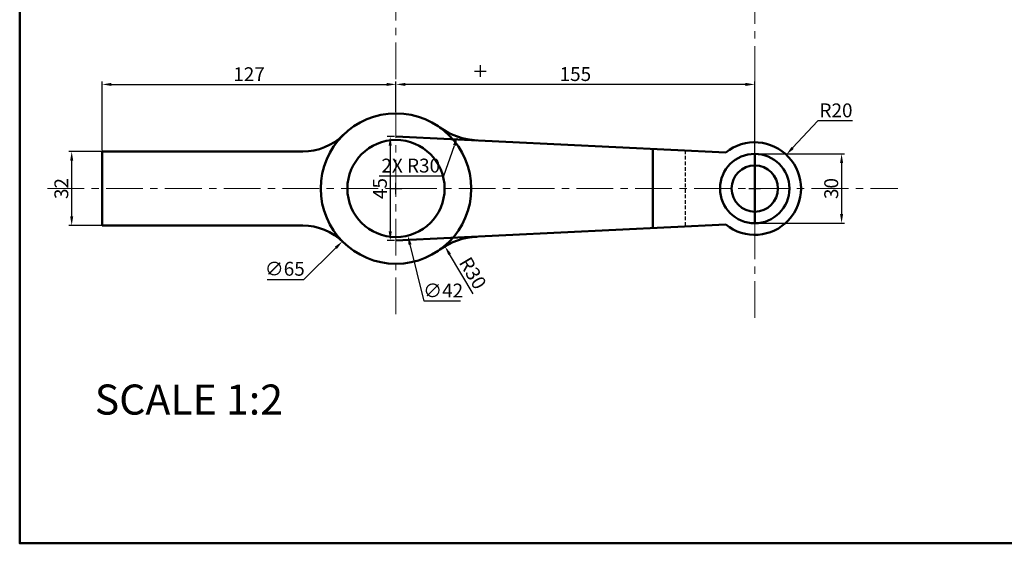
# Model space of a CAD drawing. Units: millimetres. Extents: x -1099 to -222, y 37 to 495.
# Tile 1 of 3: x -1099 to -674, y 37 to 263. Entities that reach past the tile are written whole.
import ezdxf

# ---------------------------------------------------------------- set-up
doc = ezdxf.new("R2010")
doc.units = ezdxf.units.MM
doc.header["$LTSCALE"] = 0.5
doc.linetypes.add('CENTER', pattern=[50.8, 31.75, -6.35, 6.35, -6.35])
doc.linetypes.add('HIDDEN', pattern=[9.525, 6.35, -3.175])
for name, color, linetype, lineweight in [('M-CNTR', 1, 'CENTER', 18), ('M-DIMS', 2, 'Continuous', 25), ('M-HIDN', 4, 'HIDDEN', 25), ('M-OUTL', 7, 'Continuous', 50), ('M-TEXT', 7, 'Continuous', 25), ('M-TTLB', 7, 'Continuous', 50)]:
    doc.layers.add(name, color=color, linetype=linetype, lineweight=lineweight)
doc.styles.get("Standard").update_dxf_attribs({"font": 'arial.ttf'})
doc.dimstyles.new('ISO-25', dxfattribs={"dimtxt": 6, "dimasz": 4, "dimexe": 1.25, "dimexo": 0.625, "dimtad": 1, "dimtoh": 1, "dimtxsty": 'Standard', "dimcen": 2.5, "dimadec": 0, "dimazin": 0, "dimtfac": 1, "dimtofl": 0, "dimtmove": 0, "dimatfit": 3, "dimfxl": 1, "dimarcsym": 0})

# ---------------------------------------------------------------- blocks, each defined once
blk = doc.blocks.new('*D1')
at = {"layer": 'Defpoints', "color": 0, "transparency": 16777216}
for p in [(-936.42, 234.94), (-936.42, 222.43), (-1063.42, 205.93)]:
    blk.add_point(p, dxfattribs=at)
at = {"layer": 'M-DIMS', "color": 0, "lineweight": -2, "transparency": 16777216}
for p, q in [((-1063.42, 206.56), (-1063.42, 236.19)), ((-1059.42, 234.94), (-940.42, 234.94)), ((-936.42, 223.06), (-936.42, 236.19))]:
    blk.add_line(p, q, dxfattribs=at)
at = {"layer": 'M-DIMS', "color": 0, "transparency": 16777216}
for points in [[(-1059.42, 235.6), (-1059.42, 234.27), (-1063.42, 234.94)], [(-940.42, 235.6), (-940.42, 234.27), (-936.42, 234.94)]]:
    blk.add_solid(points, dxfattribs=at)
at = {"layer": 'M-DIMS', "color": 0, "transparency": 16777216, "insert": (-999.92, 238.57), "char_height": 6, "attachment_point": 5}
blk.add_mtext('127', dxfattribs=at)
blk = doc.blocks.new('*D2')
at = {"layer": 'Defpoints', "color": 0, "transparency": 16777216}
for p in [(-936.42, 234.94), (-936.42, 222.43), (-781.42, 189.93)]:
    blk.add_point(p, dxfattribs=at)
at = {"layer": 'M-DIMS', "color": 0, "lineweight": -2, "transparency": 16777216}
for p, q in [((-936.42, 223.06), (-936.42, 236.19)), ((-785.42, 234.94), (-932.42, 234.94)), ((-781.42, 190.56), (-781.42, 236.19))]:
    blk.add_line(p, q, dxfattribs=at)
at = {"layer": 'M-DIMS', "color": 0, "transparency": 16777216}
for points in [[(-932.42, 235.6), (-932.42, 234.27), (-936.42, 234.94)], [(-785.42, 235.6), (-785.42, 234.27), (-781.42, 234.94)]]:
    blk.add_solid(points, dxfattribs=at)
at = {"layer": 'M-DIMS', "color": 0, "transparency": 16777216, "insert": (-858.92, 238.63), "char_height": 6, "attachment_point": 5}
blk.add_mtext('155', dxfattribs=at)
blk = doc.blocks.new('*D3')
at = {"layer": 'Defpoints', "color": 0, "transparency": 16777216}
for p in [(-936.42, 212.43), (-938.92, 167.43), (-936.42, 167.43)]:
    blk.add_point(p, dxfattribs=at)
at = {"layer": 'M-DIMS', "color": 0, "lineweight": -2, "transparency": 16777216}
for p, q in [((-937.04, 212.43), (-940.17, 212.43)), ((-938.92, 208.43), (-938.92, 171.43)), ((-937.04, 167.43), (-940.17, 167.43))]:
    blk.add_line(p, q, dxfattribs=at)
at = {"layer": 'M-DIMS', "color": 0, "transparency": 16777216}
for points in [[(-939.59, 208.43), (-938.25, 208.43), (-938.92, 212.43)], [(-939.59, 171.43), (-938.25, 171.43), (-938.92, 167.43)]]:
    blk.add_solid(points, dxfattribs=at)
at = {"layer": 'M-DIMS', "color": 0, "transparency": 16777216, "insert": (-942.6, 189.93), "char_height": 6, "attachment_point": 5, "rotation": 90}
blk.add_mtext('45', dxfattribs=at)
blk = doc.blocks.new('*D4')
at = {"layer": 'Defpoints', "color": 0, "transparency": 16777216}
for p in [(-941.53, 210.3), (-931.31, 169.56)]:
    blk.add_point(p, dxfattribs=at)
at = {"layer": 'M-DIMS', "color": 0, "lineweight": -2, "transparency": 16777216}
for p, q in [((-936.42, 187.43), (-936.42, 192.43)), ((-938.92, 189.93), (-933.92, 189.93)), ((-924.19, 141.2), (-930.33, 165.68)), ((-908.5, 141.2), (-924.19, 141.2))]:
    blk.add_line(p, q, dxfattribs=at)
at = {"layer": 'M-DIMS', "color": 0, "transparency": 16777216}
blk.add_solid([(-929.69, 165.85), (-930.98, 165.52), (-931.31, 169.56)], dxfattribs=at)
at = {"layer": 'M-DIMS', "color": 0, "transparency": 16777216, "insert": (-916.04, 145.06), "char_height": 6, "attachment_point": 5}
blk.add_mtext('∅42', dxfattribs=at)
blk = doc.blocks.new('*D5')
at = {"layer": 'Defpoints', "color": 0, "transparency": 16777216}
for p in [(-913.28, 212.76), (-959.56, 167.11)]:
    blk.add_point(p, dxfattribs=at)
at = {"layer": 'M-DIMS', "color": 0, "lineweight": -2, "transparency": 16777216}
for p, q in [((-936.42, 187.43), (-936.42, 192.43)), ((-938.92, 189.93), (-933.92, 189.93)), ((-976.27, 150.62), (-962.4, 164.3)), ((-992.06, 150.62), (-976.27, 150.62))]:
    blk.add_line(p, q, dxfattribs=at)
at = {"layer": 'M-DIMS', "color": 0, "transparency": 16777216}
blk.add_solid([(-962.87, 164.77), (-961.94, 163.82), (-959.56, 167.11)], dxfattribs=at)
at = {"layer": 'M-DIMS', "color": 0, "transparency": 16777216, "insert": (-984.48, 154.47), "char_height": 6, "attachment_point": 5}
blk.add_mtext('∅65', dxfattribs=at)
blk = doc.blocks.new('*D6')
at = {"layer": 'Defpoints', "color": 0, "transparency": 16777216}
for p in [(-767.79, 204.56), (-781.42, 189.93)]:
    blk.add_point(p, dxfattribs=at)
at = {"layer": 'M-DIMS', "color": 0, "lineweight": -2, "transparency": 16777216}
for p, q in [((-754.09, 219.26), (-765.06, 207.49)), ((-739.15, 219.26), (-754.09, 219.26)), ((-781.42, 187.43), (-781.42, 192.43)), ((-783.92, 189.93), (-778.92, 189.93))]:
    blk.add_line(p, q, dxfattribs=at)
at = {"layer": 'M-DIMS', "color": 0, "transparency": 16777216}
blk.add_solid([(-765.55, 207.94), (-764.57, 207.04), (-767.79, 204.56)], dxfattribs=at)
at = {"layer": 'M-DIMS', "color": 0, "transparency": 16777216, "insert": (-746.31, 222.95), "char_height": 6, "attachment_point": 5}
blk.add_mtext('R20', dxfattribs=at)
blk = doc.blocks.new('*D7')
at = {"layer": 'Defpoints', "color": 0, "transparency": 16777216}
for p in [(-1076.54, 205.93), (-1032.31, 205.93), (-1032.31, 173.93)]:
    blk.add_point(p, dxfattribs=at)
at = {"layer": 'M-DIMS', "color": 0, "lineweight": -2, "transparency": 16777216}
for p, q in [((-1032.93, 205.93), (-1077.79, 205.93)), ((-1076.54, 177.93), (-1076.54, 201.93)), ((-1032.93, 173.93), (-1077.79, 173.93))]:
    blk.add_line(p, q, dxfattribs=at)
at = {"layer": 'M-DIMS', "color": 0, "transparency": 16777216}
for points in [[(-1077.2, 201.93), (-1075.87, 201.93), (-1076.54, 205.93)], [(-1077.2, 177.93), (-1075.87, 177.93), (-1076.54, 173.93)]]:
    blk.add_solid(points, dxfattribs=at)
at = {"layer": 'M-DIMS', "color": 0, "transparency": 16777216, "insert": (-1080.23, 189.93), "char_height": 6, "attachment_point": 5, "rotation": 90}
blk.add_mtext('32', dxfattribs=at)
blk = doc.blocks.new('*D35')
at = {"layer": 'Defpoints', "color": 0, "ltscale": 0.5, "transparency": 16777216}
for p in [(-781.42, 204.93), (-781.42, 174.93), (-743.9, 174.93)]:
    blk.add_point(p, dxfattribs=at)
at = {"layer": 'M-DIMS', "color": 0, "lineweight": -2, "ltscale": 0.5, "transparency": 16777216}
for p, q in [((-780.79, 204.93), (-742.65, 204.93)), ((-743.9, 200.93), (-743.9, 178.93)), ((-780.79, 174.93), (-742.65, 174.93))]:
    blk.add_line(p, q, dxfattribs=at)
at = {"layer": 'M-DIMS', "color": 0, "ltscale": 0.5, "transparency": 16777216}
for points in [[(-744.56, 200.93), (-743.23, 200.93), (-743.9, 204.93)], [(-744.56, 178.93), (-743.23, 178.93), (-743.9, 174.93)]]:
    blk.add_solid(points, dxfattribs=at)
at = {"layer": 'M-DIMS', "color": 0, "ltscale": 0.5, "transparency": 16777216, "insert": (-747.59, 189.93), "char_height": 6, "attachment_point": 5, "rotation": 90}
blk.add_mtext('30', dxfattribs=at)
blk = doc.blocks.new('*D36')
at = {"layer": 'Defpoints', "color": 0, "ltscale": 0.5, "transparency": 16777216}
for p in [(-915.29, 164.95), (-899.97, 139.16)]:
    blk.add_point(p, dxfattribs=at)
at = {"layer": 'M-DIMS', "color": 0, "lineweight": -2, "ltscale": 0.5, "transparency": 16777216}
blk.add_line((-903.09, 144.4), (-913.25, 161.51), dxfattribs=at)
at = {"layer": 'M-DIMS', "color": 0, "ltscale": 0.5, "transparency": 16777216}
blk.add_solid([(-912.68, 161.85), (-913.82, 161.17), (-915.29, 164.95)], dxfattribs=at)
at = {"layer": 'M-DIMS', "color": 0, "ltscale": 0.5, "transparency": 16777216, "insert": (-903.89, 152.98), "char_height": 6, "attachment_point": 5, "rotation": 300.714}
blk.add_mtext('R30', dxfattribs=at)
blk = doc.blocks.new('*D49')
at = {"layer": 'Defpoints', "color": 0, "ltscale": 0.5, "transparency": 16777216}
for p in [(-899.97, 240.7), (-909.85, 212.37)]:
    blk.add_point(p, dxfattribs=at)
at = {"layer": 'M-DIMS', "color": 0, "lineweight": -2, "ltscale": 0.5, "transparency": 16777216}
for p, q in [((-899.97, 238.2), (-899.97, 243.2)), ((-902.47, 240.7), (-897.47, 240.7)), ((-915.77, 195.38), (-911.16, 208.6)), ((-943.71, 195.38), (-915.77, 195.38))]:
    blk.add_line(p, q, dxfattribs=at)
at = {"layer": 'M-DIMS', "color": 0, "ltscale": 0.5, "transparency": 16777216}
blk.add_solid([(-911.79, 208.82), (-910.54, 208.38), (-909.85, 212.37)], dxfattribs=at)
at = {"layer": 'M-DIMS', "color": 0, "ltscale": 0.5, "transparency": 16777216, "insert": (-930.05, 199.07), "char_height": 6, "attachment_point": 5}
blk.add_mtext('2X R30', dxfattribs=at)

msp = doc.modelspace()

# ---------------------------------------------------------------- linework, layer by layer
at = {"layer": 'M-CNTR'}
for p, q in [((-936.42, 135.602), (-936.42, 379.969)), ((-781.42, 134.066), (-781.42, 374.873)), ((-1087.05, 189.931), (-719.619, 189.931))]:
    msp.add_line(p, q, dxfattribs=at)
at = {"layer": 'M-HIDN', "ltscale": 0.5}
msp.add_line((-811.42, 206.383), (-811.42, 173.479), dxfattribs=at)
at = {"layer": 'M-OUTL'}
for p, q in [((-936.42, 212.431), (-793.929, 205.536)), ((-903.92, 210.858), (-903.92, 210.963)), ((-1063.42, 205.931), (-1063.42, 173.931)), ((-1063.42, 205.931), (-976.734, 205.931)), ((-1063.42, 173.931), (-976.734, 173.931)), ((-793.929, 174.326), (-936.42, 167.431))]:
    msp.add_line(p, q, dxfattribs=at)
at = {"layer": 'M-OUTL', "ltscale": 0.5}
for p, q in [((-825.42, 207.06), (-825.42, 172.802)), ((-781.42, 204.931), (-781.42, 174.931))]:
    msp.add_line(p, q, dxfattribs=at)
at = {"layer": 'M-OUTL'}
for centre, radius in [((-936.42, 189.931), 32.5), ((-936.42, 189.931), 21), ((-781.42, 189.931), 15), ((-781.42, 189.931), 10)]:
    msp.add_circle(centre, radius, dxfattribs=at)
for centre, radius, start, end in [((-976.734, 230.931), 25, 270, 314.51692), ((-899.971, 240.702), 30, 234.32551, 267.22978), ((-781.42, 189.931), 20, 231.28473, 128.71527), ((-976.734, 148.931), 25, 45.48308, 90), ((-899.971, 139.16), 30, 92.77022, 125.67449)]:
    msp.add_arc(centre, radius, start, end, dxfattribs=at)
at = {"layer": 'M-TTLB', "ltscale": 0.5}
msp.add_lwpolyline([(-1099.005, 495.37), (-222.205, 495.37), (-222.205, 36.581), (-1099.005, 36.581)], close=True, dxfattribs=at)

# ---------------------------------------------------------------- texts
at = {"layer": 'M-TEXT', "ltscale": 0.5, "insert": (-1066.574, 105.219), "char_height": 13, "attachment_point": 1}
msp.add_mtext_dynamic_manual_height_columns('SCALE 1:2', width=90.11386, gutter_width=12.5, heights=[0], dxfattribs=at)

# ---------------------------------------------------------------- dimensions: what is measured, and where the dimension line sits
at = {"layer": 'M-DIMS'}
for p1, picture, middle in [((-1063.42, 205.931), '*D1', (-999.92, 238.575)), ((-781.42, 189.931), '*D2', (-858.92, 238.626))]:
    dim = msp.add_linear_dim(base=(-936.42, 234.938), p1=p1, p2=(-936.42, 222.431), dimstyle='ISO-25', override={"dimclrd": 0, "dimclre": 0, "dimclrt": 0}, dxfattribs=at)
    dim.commit()
    dim.dimension.update_dxf_attribs({"geometry": picture, "text_midpoint": middle})
at = {"layer": 'M-DIMS', "ltscale": 0.5}
dim = msp.add_radius_dim(center=(-899.971, 240.702), mpoint=(-909.848, 212.375), text='2X <>', dimstyle='ISO-25', override={"dimdec": 0, "dimlfac": 1, "dimrnd": 0, "dimzin": 0, "dimdsep": 46, "dimlunit": 2}, dxfattribs=at)
dim.commit()
dim.dimension.update_dxf_attribs({"geometry": '*D49', "text_midpoint": (-930.055, 195.379), "dimtype": 164})
at = {"layer": 'M-DIMS'}
dim = msp.add_radius_dim(center=(-781.42, 189.931), mpoint=(-767.786, 204.564), dimstyle='ISO-25', override={"dimclrd": 0, "dimclre": 0, "dimclrt": 0}, dxfattribs=at)
dim.commit()
dim.dimension.update_dxf_attribs({"geometry": '*D6', "text_midpoint": (-746.31, 219.26), "dimtype": 164})
for p1, p2, picture, middle in [((-913.283, 212.755), (-959.556, 167.107), '*D5', (-984.478, 150.618)), ((-941.531, 210.299), (-931.308, 169.563), '*D4', (-916.036, 141.202))]:
    dim = msp.add_diameter_dim_2p(p1=p1, p2=p2, dimstyle='ISO-25', override={"dimclrd": 0, "dimclre": 0, "dimclrt": 0}, dxfattribs=at)
    dim.commit()
    dim.dimension.update_dxf_attribs({"geometry": picture, "text_midpoint": middle, "dimtype": 163})
for base, p1, p2, picture, middle in [((-938.92, 167.431), (-936.42, 212.431), (-936.42, 167.431), '*D3', (-938.92, 189.931)), ((-1076.536, 205.931), (-1032.306, 173.931), (-1032.306, 205.931), '*D7', (-1076.536, 189.931))]:
    dim = msp.add_linear_dim(base=base, p1=p1, p2=p2, angle=90, dimstyle='ISO-25', override={"dimclrd": 0, "dimclre": 0, "dimclrt": 0}, dxfattribs=at)
    dim.commit()
    dim.dimension.update_dxf_attribs({"geometry": picture, "text_midpoint": middle, "dimtype": 160})
at = {"layer": 'M-DIMS', "ltscale": 0.5}
dim = msp.add_linear_dim(base=(-743.897, 174.931), p1=(-781.42, 204.931), p2=(-781.42, 174.931), angle=90, dimstyle='ISO-25', override={"dimclrd": 0, "dimclre": 0, "dimclrt": 0}, dxfattribs=at)
dim.commit()
dim.dimension.update_dxf_attribs({"geometry": '*D35', "text_midpoint": (-747.587, 189.931)})
dim = msp.add_radius_dim(center=(-899.971, 139.16), mpoint=(-915.294, 164.951), dimstyle='ISO-25', override={"dimclrd": 0, "dimclre": 0, "dimclrt": 0}, dxfattribs=at)
dim.commit()
dim.dimension.update_dxf_attribs({"geometry": '*D36', "text_midpoint": (-907.06, 151.093), "dimtype": 164})

doc.saveas('drawing.dxf')
